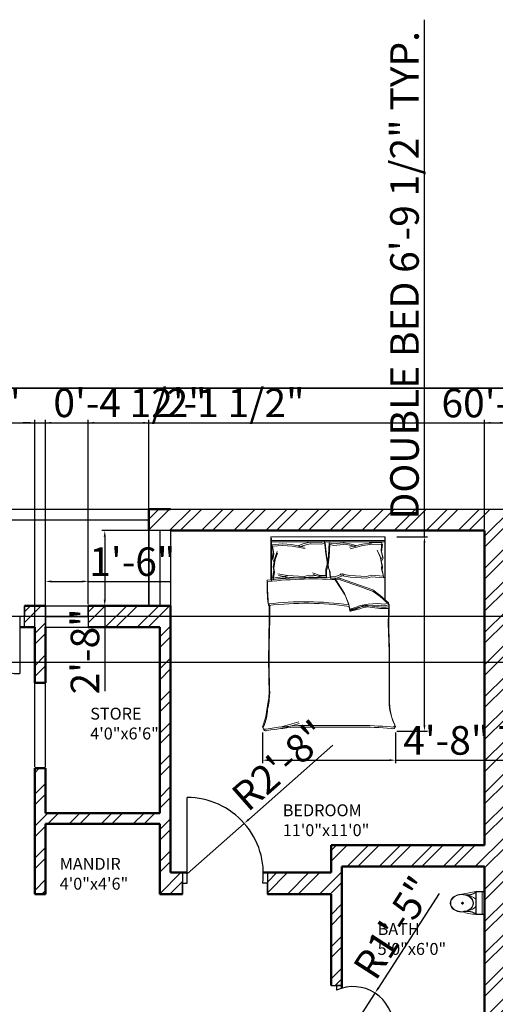
# Model space of a CAD drawing. Units: inches. Extents: x 1990 to 2869, y 1755 to 2533.
# Tile 3 of 6: x 2216 to 2415, y 2120 to 2533. Entities that reach past the tile are written whole.
import ezdxf

# ---------------------------------------------------------------- set-up
doc = ezdxf.new("R2010")
doc.units = ezdxf.units.IN
for name, color, linetype, lineweight in [('A-ANNO-DIMS', 171, 'Continuous', 18), ('A-ANNO-TTLB', 7, 'Continuous', 35), ('A-AREA-IDEN', 7, 'Continuous', 18), ('A-DOOR', 11, 'Continuous', 25), ('A-FLOR-FIXT', 9, 'Continuous', 20), ('A-FURN', 8, 'Continuous', 18), ('A-GLAZ', 121, 'Continuous', 25), ('A-WALL', 7, 'Continuous', 50), ('A-WALL-SITE', 7, 'Continuous', 30)]:
    doc.layers.add(name, color=color, linetype=linetype, lineweight=lineweight)
doc.layers.add('A-WALL-PATT', color=215, linetype='Continuous', lineweight=13, true_color=0xa953a0)
doc.styles.get("Standard").update_dxf_attribs({"font": 'arial.ttf'})
doc.dimstyles.new('ISO-25', dxfattribs={"dimtxt": 12, "dimasz": 2.5, "dimexe": 1.25, "dimexo": 0.625, "dimtad": 1, "dimdec": 0, "dimlunit": 3, "dimtxsty": 'Standard', "dimcen": 2.5, "dimadec": 0, "dimazin": 0, "dimtfac": 1, "dimtdec": 0, "dimtmove": 0, "dimatfit": 3, "dimfxl": 1, "dimarcsym": 0})

# ---------------------------------------------------------------- blocks, each defined once
blk = doc.blocks.new('A$C31115884')
for p, q in [((283, 498), (223, 498)), ((258, 466), (258, 523)), ((0, 200), (0, 0)), ((520, 200), (0, 200)), ((510, 54), (0, 54)), ((10, 190), (10, 10)), ((510, 190), (10, 190)), ((10, 10), (510, 10)), ((510, 10), (510, 190)), ((520, 0), (520, 200)), ((0, 0), (520, 0))]:
    blk.add_line(p, q)
blk.add_circle((256, 496), 23.6)
for centre, radius, start, end in [((2778, -205), 2807, 165.4549, 171.7133), ((-295, 403), 365, 324.2091, 9.3499), ((-295, 403), 375, 324.2091, 9.3499), ((806, 403), 365, 170.6501, 215.7909), ((3237, 905), 2807, 188.2867, 194.5451), ((384, 406), 293, 190.2774, 224.1564), ((139, 406), 293, 315.8436, 2.6563), ((806, 403), 375, 179.2036, 215.7909)]:
    blk.add_arc(centre, radius, start, end)
blk.add_ellipse((256, 510), major_axis=(0, -261), ratio=0.772727)
blk.add_open_spline([(256, 259), (263, 259), (270, 260), (288, 262), (299, 265), (320, 273), (330, 278), (350, 291), (360, 299), (378, 316), (386, 326), (402, 347), (409, 358), (421, 383), (427, 395), (436, 422), (440, 436), (445, 465), (447, 480), (448, 509), (448, 524), (445, 553), (443, 568), (436, 596), (432, 610), (422, 636), (416, 649), (402, 672), (395, 683), (379, 703), (370, 712), (351, 728), (341, 735), (321, 746), (310, 751), (289, 757), (278, 759), (256, 761), (245, 761), (223, 757), (212, 754), (191, 746), (181, 741), (161, 728), (151, 720), (133, 703), (125, 693), (110, 672), (103, 660), (90, 636), (85, 623), (76, 596), (72, 582), (67, 553), (66, 538), (64, 509), (65, 494), (68, 465), (70, 450), (77, 422), (81, 408), (91, 382), (97, 370), (111, 346), (118, 335), (135, 316), (144, 307), (162, 291), (172, 284), (193, 273), (203, 269), (225, 262), (236, 260), (250, 259), (253, 259), (256, 259)], degree=3, knots=[0, 0, 0, 0, 0.110105, 0.110105, 0.285049, 0.285049, 0.459994, 0.459994, 0.634938, 0.634938, 0.809882, 0.809882, 0.984827, 0.984827, 1.159771, 1.159771, 1.334715, 1.334715, 1.50966, 1.50966, 1.684604, 1.684604, 1.859549, 1.859549, 2.034493, 2.034493, 2.209437, 2.209437, 2.384382, 2.384382, 2.559326, 2.559326, 2.73427, 2.73427, 2.909215, 2.909215, 3.084159, 3.084159, 3.259103, 3.259103, 3.434048, 3.434048, 3.608992, 3.608992, 3.783936, 3.783936, 3.958881, 3.958881, 4.133825, 4.133825, 4.30877, 4.30877, 4.483714, 4.483714, 4.658658, 4.658658, 4.833603, 4.833603, 5.008547, 5.008547, 5.183491, 5.183491, 5.358436, 5.358436, 5.53338, 5.53338, 5.708324, 5.708324, 5.883269, 5.883269, 6.058213, 6.058213, 6.233158, 6.233158, 6.283185, 6.283185, 6.283185, 6.283185])
blk = doc.blocks.new('*D3')
at = {"layer": 'A-ANNO-DIMS', "color": 0, "lineweight": -2, "transparency": 16777216}
for p, q in [((2269.35, 2319.05), (2250.15, 2319.05)), ((2251.4, 2316.55), (2251.4, 2290.05)), ((2269.35, 2287.55), (2250.15, 2287.55)), ((2251.4, 2287.55), (2251.4, 2251.7))]:
    blk.add_line(p, q, dxfattribs=at)
at = {"layer": 'A-ANNO-DIMS', "color": 0, "transparency": 16777216}
for points in [[(2250.98, 2316.55), (2251.81, 2316.55), (2251.4, 2319.05)], [(2250.98, 2290.05), (2251.81, 2290.05), (2251.4, 2287.55)]]:
    blk.add_solid(points, dxfattribs=at)
at = {"layer": 'Defpoints', "color": 0, "transparency": 16777216}
for p in [(2269.97, 2319.05), (2251.4, 2287.55), (2269.97, 2287.55)]:
    blk.add_point(p, dxfattribs=at)
at = {"layer": 'A-ANNO-DIMS', "color": 0, "transparency": 16777216, "insert": (2244.64, 2268.37), "char_height": 12, "attachment_point": 5, "rotation": 90}
blk.add_mtext('2\'-8"', dxfattribs=at)
blk = doc.blocks.new('*D4')
at = {"layer": 'A-ANNO-DIMS', "color": 0, "lineweight": -2, "transparency": 16777216}
for p, q in [((2226.47, 2288.18), (2226.47, 2299)), ((2228.97, 2297.75), (2241.97, 2297.75)), ((2244.47, 2288.18), (2244.47, 2299)), ((2244.47, 2297.75), (2278.99, 2297.75))]:
    blk.add_line(p, q, dxfattribs=at)
at = {"layer": 'A-ANNO-DIMS', "color": 0, "transparency": 16777216}
for points in [[(2228.97, 2298.17), (2228.97, 2297.33), (2226.47, 2297.75)], [(2241.97, 2298.17), (2241.97, 2297.33), (2244.47, 2297.75)]]:
    blk.add_solid(points, dxfattribs=at)
at = {"layer": 'Defpoints', "color": 0, "transparency": 16777216}
for p in [(2244.47, 2297.75), (2226.47, 2287.55), (2244.47, 2287.55)]:
    blk.add_point(p, dxfattribs=at)
at = {"layer": 'A-ANNO-DIMS', "color": 0, "transparency": 16777216, "insert": (2262.98, 2304.5), "char_height": 12, "attachment_point": 5}
blk.add_mtext('1\'-6"', dxfattribs=at)
blk = doc.blocks.new('BED-DOUBLE')
for p, q in [((3.47, 63.33), (3.47, 81.44)), ((3.47, 81.44), (51.49, 81.44)), ((3.47, 79.91), (51.27, 79.91)), ((3.48, 63.33), (3.48, 81.44)), ((3.48, 79.91), (51.27, 79.91)), ((3.7, 62.69), (3.7, 80.8)), ((3.7, 62.69), (3.7, 80.8)), ((3.7, 79.27), (51.49, 79.27)), ((3.7, 79.27), (51.49, 79.27)), ((16.88, 78.42), (19.77, 79.14)), ((16.88, 78.42), (19.77, 79.14)), ((19.77, 79.14), (20.09, 79.14)), ((19.77, 79.14), (20.09, 79.14)), ((20.09, 79.14), (24.54, 78.99)), ((20.09, 79.14), (24.54, 78.99)), ((24.54, 78.99), (25.98, 79.57)), ((24.54, 78.99), (25.98, 79.57)), ((24.77, 78.36), (26.21, 78.93)), ((24.77, 78.36), (26.21, 78.93)), ((25.98, 79.57), (26.56, 74.22)), ((25.98, 79.57), (26.56, 74.22)), ((26.21, 78.93), (26.79, 73.58)), ((26.21, 78.93), (26.79, 73.58)), ((27.98, 78.95), (27.73, 73.58)), ((27.98, 78.95), (27.73, 73.58)), ((29.46, 78.46), (27.98, 78.95)), ((29.46, 78.46), (27.98, 78.95)), ((33.88, 78.89), (29.46, 78.46)), ((33.88, 78.89), (29.46, 78.46)), ((34.2, 78.91), (33.88, 78.89)), ((34.2, 78.91), (33.88, 78.89)), ((37.14, 78.36), (34.2, 78.91)), ((37.13, 78.36), (34.2, 78.91)), ((45.71, 78.9), (41.91, 78.37)), ((45.71, 78.9), (41.91, 78.37)), ((50.11, 78.89), (44.71, 78.98)), ((44.71, 78.98), (45.71, 78.9)), ((50.11, 78.89), (44.71, 78.98)), ((44.71, 78.98), (45.71, 78.9)), ((50.11, 78.89), (49.73, 75.68)), ((50.11, 78.89), (49.73, 75.68)), ((51.27, 81.44), (51.27, 54.83)), ((51.27, 81.44), (51.27, 54.83)), ((51.49, 81.44), (51.49, 80.8)), ((51.49, 80.8), (51.49, 54.19)), ((51.49, 80.8), (51.49, 54.19)), ((3.89, 78.13), (4.47, 74.95)), ((3.89, 78.13), (4.47, 74.95)), ((3.9, 78.11), (8.18, 78.43)), ((3.9, 78.11), (8.18, 78.43)), ((4.47, 74.95), (4.04, 72.34)), ((4.47, 74.95), (4.04, 72.34)), ((4.12, 77.49), (4.7, 74.31)), ((4.12, 77.49), (4.7, 74.31)), ((4.13, 77.47), (8.41, 77.8)), ((4.13, 77.47), (8.41, 77.8)), ((5.05, 72.49), (6.06, 75.24)), ((5.05, 72.49), (6.06, 75.24)), ((5.28, 71.85), (6.29, 74.6)), ((5.28, 71.85), (6.29, 74.6)), ((8.18, 78.43), (8.28, 78.42)), ((8.18, 78.43), (8.28, 78.42)), ((8.28, 78.42), (12.11, 78.13)), ((8.28, 78.42), (12.11, 78.13)), ((8.41, 77.8), (8.51, 77.78)), ((8.41, 77.8), (8.51, 77.78)), ((8.51, 77.78), (12.34, 77.49)), ((8.51, 77.78), (12.34, 77.49)), ((12.11, 78.13), (17.6, 77.11)), ((12.11, 78.13), (17.6, 77.11)), ((12.34, 77.49), (17.83, 76.48)), ((12.34, 77.49), (17.83, 76.48)), ((14.85, 77.69), (16.88, 78.42)), ((14.85, 77.69), (16.88, 78.42)), ((15.08, 77.05), (17.11, 77.78)), ((15.08, 77.05), (17.11, 77.78)), ((17.11, 77.78), (20, 78.5)), ((17.11, 77.78), (20, 78.5)), ((20, 78.5), (20.32, 78.5)), ((20, 78.5), (20.32, 78.5)), ((20.32, 78.5), (24.77, 78.36)), ((20.32, 78.5), (24.77, 78.36)), ((28.21, 78.31), (27.96, 72.94)), ((28.2, 78.31), (27.96, 72.94)), ((29.68, 77.82), (28.2, 78.31)), ((29.68, 77.82), (28.21, 78.31)), ((34.11, 78.25), (29.68, 77.82)), ((34.11, 78.25), (29.68, 77.82)), ((34.43, 78.27), (34.11, 78.25)), ((34.43, 78.27), (34.11, 78.25)), ((37.36, 77.73), (34.43, 78.27)), ((37.36, 77.73), (34.43, 78.27)), ((41.91, 78.37), (36.49, 77.02)), ((41.91, 78.37), (36.49, 77.02)), ((42.14, 77.73), (36.72, 76.38)), ((42.14, 77.73), (36.72, 76.38)), ((39.2, 77.77), (37.13, 78.36)), ((39.2, 77.77), (37.14, 78.36)), ((39.43, 77.13), (37.36, 77.73)), ((39.43, 77.13), (37.36, 77.73)), ((45.94, 78.26), (42.14, 77.73)), ((45.94, 78.26), (42.14, 77.73)), ((50.34, 78.25), (44.94, 78.34)), ((44.94, 78.34), (45.94, 78.26)), ((50.34, 78.25), (44.94, 78.34)), ((44.94, 78.34), (45.94, 78.26)), ((49.31, 73.19), (48.13, 75.86)), ((49.31, 73.19), (48.13, 75.86)), ((49.54, 72.55), (48.36, 75.23)), ((49.54, 72.55), (48.36, 75.23)), ((49.73, 75.68), (50.33, 73.1)), ((49.73, 75.68), (50.33, 73.1)), ((50.34, 78.25), (49.96, 75.04)), ((50.34, 78.25), (49.96, 75.04)), ((49.96, 75.04), (50.56, 72.47)), ((49.96, 75.04), (50.56, 72.47)), ((4.04, 72.34), (4.62, 71.33)), ((4.04, 72.34), (4.62, 71.33)), ((4.7, 74.31), (4.27, 71.7)), ((4.7, 74.31), (4.27, 71.7)), ((4.27, 71.7), (4.85, 70.69)), ((4.27, 71.7), (4.85, 70.69)), ((4.47, 68.87), (5.05, 72.49)), ((4.47, 68.87), (5.05, 72.49)), ((4.7, 68.23), (5.28, 71.85)), ((4.7, 68.23), (5.28, 71.85)), ((26.56, 74.22), (27.14, 71.04)), ((26.56, 74.22), (27.14, 71.04)), ((26.79, 73.58), (27.37, 70.4)), ((26.79, 73.58), (27.37, 70.4)), ((27.14, 71.04), (27.14, 69.74)), ((27.14, 71.04), (27.14, 69.74)), ((27.73, 73.58), (27.35, 70.37)), ((27.73, 73.58), (27.35, 70.37)), ((27.35, 70.37), (27.44, 69.07)), ((27.35, 70.37), (27.44, 69.07)), ((27.37, 70.4), (27.37, 69.1)), ((27.37, 70.4), (27.37, 69.1)), ((27.96, 72.94), (27.58, 69.73)), ((27.96, 72.94), (27.58, 69.73)), ((50.11, 69.61), (49.31, 73.19)), ((50.11, 69.61), (49.31, 73.19)), ((50.34, 68.98), (49.54, 72.55)), ((50.34, 68.98), (49.54, 72.55)), ((50.33, 73.1), (49.81, 72.06)), ((50.33, 73.1), (49.81, 72.06)), ((50.56, 72.47), (50.04, 71.42)), ((50.56, 72.47), (50.04, 71.42)), ((4.18, 64.1), (4.76, 67.28)), ((4.18, 64.1), (4.76, 67.28)), ((4.41, 63.46), (4.99, 66.64)), ((4.41, 63.46), (4.99, 66.64)), ((4.76, 67.28), (4.47, 68.87)), ((4.76, 67.28), (4.47, 68.87)), ((4.99, 66.64), (4.7, 68.23)), ((4.99, 66.64), (4.7, 68.23)), ((24.1, 65.18), (20.96, 66.27)), ((24.1, 65.18), (20.96, 66.27)), ((27.14, 69.74), (26.56, 67.86)), ((27.14, 69.74), (26.56, 67.86)), ((26.56, 67.86), (26.56, 65.18)), ((26.56, 67.86), (26.56, 65.18)), ((27.37, 69.1), (26.79, 67.22)), ((27.37, 69.1), (26.79, 67.22)), ((26.79, 67.22), (26.79, 64.54)), ((26.79, 67.22), (26.79, 64.54)), ((27.44, 69.07), (28.13, 67.23)), ((27.44, 69.07), (28.13, 67.23)), ((27.58, 69.73), (27.66, 68.43)), ((27.58, 69.73), (27.66, 68.43)), ((27.66, 68.43), (28.36, 66.59)), ((27.66, 68.43), (28.36, 66.59)), ((28.13, 67.23), (28.3, 64.55)), ((28.13, 67.23), (28.3, 64.55)), ((28.36, 66.59), (28.53, 63.91)), ((28.36, 66.59), (28.53, 63.91)), ((49.92, 68.01), (50.11, 69.61)), ((49.92, 68.01), (50.11, 69.61)), ((50.7, 64.87), (49.92, 68.01)), ((50.7, 64.87), (49.92, 68.01)), ((50.15, 67.37), (50.34, 68.98)), ((50.15, 67.37), (50.34, 68.98)), ((50.93, 64.23), (50.15, 67.37)), ((50.93, 64.23), (50.15, 67.37)), ((9.28, 64.82), (4.18, 64.1)), ((9.28, 64.82), (4.18, 64.1)), ((9.51, 64.19), (4.41, 63.46)), ((9.51, 64.19), (4.41, 63.46)), ((6.38, 65.81), (10.41, 65.15)), ((6.38, 65.81), (10.41, 65.15)), ((6.61, 65.18), (10.64, 64.51)), ((6.61, 65.18), (10.64, 64.51)), ((10.41, 65.15), (9.28, 64.82)), ((10.41, 65.15), (9.28, 64.82)), ((10.64, 64.51), (9.51, 64.19)), ((10.64, 64.51), (9.51, 64.19)), ((10.41, 65.15), (17.42, 64.72)), ((10.41, 65.15), (17.42, 64.72)), ((10.64, 64.51), (17.65, 64.08)), ((10.64, 64.51), (17.65, 64.08)), ((17.42, 64.72), (19.38, 65.27)), ((17.42, 64.72), (19.38, 65.27)), ((17.65, 64.08), (19.61, 64.63)), ((17.65, 64.08), (19.61, 64.63)), ((19.38, 65.27), (24.52, 64.87)), ((19.38, 65.27), (24.52, 64.87)), ((19.61, 64.63), (24.74, 64.23)), ((19.61, 64.63), (24.74, 64.23)), ((24.33, 64.54), (21.19, 65.63)), ((24.33, 64.54), (21.19, 65.63)), ((26.56, 65.18), (24.1, 65.18)), ((26.56, 65.18), (24.1, 65.18)), ((26.79, 64.54), (24.33, 64.54)), ((26.79, 64.54), (24.33, 64.54)), ((28.3, 64.55), (30.75, 64.7)), ((28.3, 64.55), (30.75, 64.7)), ((28.53, 63.91), (30.98, 64.06)), ((28.53, 63.91), (30.98, 64.06)), ((30.26, 64.06), (34.45, 57.57)), ((30.26, 64.06), (34.45, 57.57)), ((30.49, 63.42), (34.68, 56.93)), ((30.49, 63.42), (34.68, 56.93)), ((30.75, 64.7), (33.82, 65.99)), ((30.75, 64.7), (33.82, 65.99)), ((30.98, 64.06), (34.05, 65.35)), ((30.98, 64.06), (34.05, 65.35)), ((40.64, 61.13), (32.31, 64.06)), ((40.64, 61.13), (32.31, 64.06)), ((40.87, 60.49), (32.53, 63.42)), ((40.87, 60.49), (32.53, 63.42)), ((32.56, 65.81), (36.6, 65.15)), ((32.56, 65.81), (36.6, 65.15)), ((32.79, 65.18), (36.82, 64.51)), ((32.79, 65.18), (36.82, 64.51)), ((36.6, 65.15), (43.61, 64.72)), ((36.6, 65.15), (43.61, 64.72)), ((36.82, 64.51), (43.83, 64.08)), ((36.82, 64.51), (43.83, 64.08)), ((43.61, 64.72), (45.57, 65.27)), ((43.61, 64.72), (45.57, 65.27)), ((43.83, 64.08), (45.79, 64.63)), ((43.83, 64.08), (45.79, 64.63)), ((45.57, 65.27), (50.7, 64.87)), ((45.57, 65.27), (50.7, 64.87)), ((45.79, 64.63), (50.93, 64.23)), ((45.79, 64.63), (50.93, 64.23)), ((46.22, 59.11), (40.64, 61.13)), ((46.22, 59.11), (40.64, 61.13)), ((46.45, 58.48), (40.87, 60.49)), ((46.45, 58.48), (40.87, 60.49)), ((49.16, 56.95), (46.22, 59.11)), ((49.16, 56.95), (46.22, 59.11)), ((49.39, 56.31), (46.45, 58.48)), ((49.39, 56.31), (46.45, 58.48)), ((34.45, 57.57), (36.15, 53.08)), ((34.45, 57.57), (36.15, 53.08)), ((34.68, 56.93), (36.38, 52.44)), ((34.68, 56.93), (36.38, 52.44)), ((52.87, 53.7), (49.16, 56.95)), ((52.87, 53.7), (49.16, 56.95)), ((53.1, 53.06), (49.39, 56.31)), ((53.1, 53.06), (49.39, 56.31)), ((36.15, 53.08), (36.46, 51.07)), ((36.15, 53.08), (36.46, 51.07)), ((36.38, 52.44), (36.69, 50.43)), ((36.38, 52.44), (36.69, 50.43)), ((36.46, 51.07), (38.94, 51.69)), ((36.46, 51.07), (38.94, 51.69)), ((36.69, 50.43), (39.17, 51.05)), ((36.69, 50.43), (39.17, 51.05)), ((38.94, 51.69), (40.95, 52.61)), ((38.94, 51.69), (40.95, 52.61)), ((39.17, 51.05), (41.18, 51.97)), ((39.17, 51.05), (41.18, 51.97)), ((40.95, 52.61), (44.36, 53.08)), ((40.95, 52.61), (44.36, 53.08)), ((41.18, 51.97), (44.59, 52.44)), ((41.18, 51.97), (44.59, 52.44)), ((44.36, 53.08), (48.23, 53.39)), ((44.36, 53.08), (48.23, 53.39)), ((44.59, 52.44), (48.46, 52.75)), ((44.59, 52.44), (48.46, 52.75)), ((48.23, 53.39), (51.33, 53.08)), ((48.23, 53.39), (51.33, 53.08)), ((48.46, 52.75), (51.56, 52.44)), ((48.46, 52.75), (51.56, 52.44)), ((51.33, 53.08), (52.87, 53.7)), ((51.33, 53.08), (52.87, 53.7)), ((51.56, 52.44), (53.1, 53.06)), ((51.56, 52.44), (53.1, 53.06)), ((52.95, 51.95), (52.87, 53.7, 3.87)), ((52.95, 51.95), (52.87, 53.7, 3.87)), ((53.18, 51.31), (53.1, 53.06, 3.87)), ((53.18, 51.31), (53.1, 53.06, 3.87)), ((15.06, 2.2), (39.68, 2.2)), ((15.06, 2.2), (39.68, 2.2)), ((15.29, 1.56), (39.91, 1.56)), ((15.29, 1.56), (39.91, 1.56))]:
    blk.add_line(p, q)
for centre, radius, start, end in [((85.16, 61.35), 83.31, 178.7218, 185.604), ((85.16, 61.35), 83.31, 178.7218, 185.604), ((21.36, -100.61), 164.97, 86.0865, 96.7821), ((21.36, -100.61), 164.97, 86.0865, 96.7821), ((85.39, 60.71), 83.31, 178.7218, 185.604), ((85.39, 60.71), 83.31, 178.7218, 185.604), ((21.59, -101.25), 164.97, 86.0865, 96.7821), ((21.59, -101.25), 164.97, 86.0865, 96.7821), ((17.76, -74.87), 129.02, 81.7845, 96.9006), ((17.76, -74.87), 129.02, 81.7845, 96.9006), ((17.98, -75.51), 129.02, 81.7845, 96.9006), ((17.98, -75.51), 129.02, 81.7845, 96.9006), ((-167.31, 50.27), 170.11, 358.4762, 1.0082), ((-167.31, 50.27), 170.11, 358.4762, 1.0082), ((-167.08, 49.63), 170.11, 358.4762, 1.0082), ((-167.08, 49.63), 170.11, 358.4762, 1.0082), ((36.64, 51), 0.185, 160.2464, 271.1377), ((36.64, 51), 0.185, 160.2464, 271.1377), ((31.15, 79.96), 29.65, 280.6617, 289.8806), ((31.15, 79.96), 29.65, 280.6617, 289.8806), ((36.86, 50.36), 0.185, 160.2464, 271.1377), ((36.86, 50.36), 0.185, 160.2464, 271.1377), ((31.38, 79.32), 29.65, 280.6617, 289.8806), ((31.38, 79.32), 29.65, 280.6617, 289.8806), ((43.74, 46.38), 6.22, 78.6608, 113.7384), ((43.74, 46.38), 6.22, 78.6608, 113.7384), ((43.97, 45.74), 6.22, 78.6608, 113.7384), ((43.97, 45.74), 6.22, 78.6608, 113.7384), ((51.33, 88.1), 36.18, 259.8763, 272.5657), ((51.33, 88.1), 36.18, 259.8763, 272.5657), ((51.56, 87.46), 36.18, 259.8763, 272.5657), ((51.56, 87.46), 36.18, 259.8763, 272.5657), ((182.27, 45.13), 129.5, 176.9791, 183.8365), ((182.27, 45.13), 129.5, 176.9791, 183.8365), ((182.49, 44.49), 129.5, 176.9791, 183.8365), ((182.49, 44.49), 129.5, 176.9791, 183.8365), ((484.82, 30.83), 482.31, 178.2277, 181.7185), ((484.82, 30.83), 482.31, 178.2277, 181.7185), ((485.05, 30.19), 482.31, 178.2277, 181.7185), ((485.05, 30.19), 482.31, 178.2277, 181.7185), ((-4508.74, 13.62), 4561.86, 0.00217, 0.28689), ((-4508.74, 13.62), 4561.86, 0.00217, 0.28689), ((-4508.52, 12.98), 4561.86, 0.00217, 0.28689), ((-4508.52, 12.98), 4561.86, 0.00217, 0.28689), ((-26.9, 16.93), 29.63, 346.0648, 358.9113), ((-26.9, 16.93), 29.63, 346.0648, 358.9113), ((-26.67, 16.29), 29.63, 346.0648, 358.9113), ((-26.67, 16.29), 29.63, 346.0648, 358.9113), ((76.16, 12.78), 23.07, 177.4714, 206.4681), ((76.16, 12.78), 23.07, 177.4714, 206.4681), ((76.39, 12.14), 23.07, 177.4714, 206.4681), ((76.39, 12.14), 23.07, 177.4714, 206.4681), ((-21.66, 11.17), 23.56, 337.9751, 356.652), ((-21.66, 11.17), 23.56, 337.9751, 356.652), ((-21.43, 10.53), 23.56, 337.9751, 356.652), ((-21.43, 10.53), 23.56, 337.9751, 356.652), ((1.09, 1.73), 1.09, 146.1736, 293.4781), ((1.09, 1.73), 1.09, 146.1736, 293.4781), ((1.32, 1.09), 1.09, 146.1736, 293.4781), ((1.32, 1.09), 1.09, 146.1736, 293.4781), ((21.43, -119.39), 121.76, 92.9958, 99.4091), ((21.43, -119.39), 121.76, 92.9958, 99.4091), ((21.66, -120.03), 121.76, 92.9958, 99.4091), ((21.65, -120.03), 121.76, 92.9958, 99.4091), ((-17.22, 105.15), 106.46, 283.3832, 287.7053), ((-17.22, 105.15), 106.46, 283.3832, 287.7053), ((-16.99, 104.52), 106.46, 283.3832, 287.7053), ((-16.99, 104.52), 106.46, 283.3832, 287.7053), ((41.15, -130.83), 133.04, 84.4998, 90.6351), ((41.15, -130.83), 133.04, 84.4998, 90.6351), ((41.38, -131.47), 133.04, 84.4998, 90.6351), ((41.38, -131.47), 133.04, 84.4998, 90.6351), ((54.41, 2.57), 1.1, 242.6588, 356.02), ((54.41, 2.57), 1.1, 242.6588, 356.02), ((54.64, 1.93), 1.1, 242.6588, 356.02), ((54.64, 1.93), 1.1, 242.6588, 356.02)]:
    blk.add_arc(centre, radius, start, end)
blk = doc.blocks.new('*D20')
at = {"layer": 'A-ANNO-DIMS', "color": 0, "lineweight": -2, "transparency": 16777216}
for p, q in [((2385.7, 2316.5), (2385.7, 2533.49)), ((2374.09, 2316.5), (2386.95, 2316.5)), ((2385.7, 2237.45), (2385.7, 2314)), ((2374.09, 2234.95), (2386.95, 2234.95))]:
    blk.add_line(p, q, dxfattribs=at)
at = {"layer": 'A-ANNO-DIMS', "color": 0, "transparency": 16777216}
for points in [[(2385.29, 2314), (2386.12, 2314), (2385.7, 2316.5)], [(2385.29, 2237.45), (2386.12, 2237.45), (2385.7, 2234.95)]]:
    blk.add_solid(points, dxfattribs=at)
at = {"layer": 'Defpoints', "color": 0, "transparency": 16777216}
for p in [(2373.47, 2316.5), (2385.7, 2316.5), (2373.47, 2234.95)]:
    blk.add_point(p, dxfattribs=at)
at = {"layer": 'A-ANNO-DIMS', "color": 0, "transparency": 16777216, "insert": (2378.87, 2426.24), "char_height": 12, "attachment_point": 5, "rotation": 90}
blk.add_mtext('DOUBLE BED 6\'-9 1/2" TYP.', dxfattribs=at)
blk = doc.blocks.new('*D21')
at = {"layer": 'A-ANNO-DIMS', "color": 0, "lineweight": -2, "transparency": 16777216}
for p, q in [((2317.65, 2234.33), (2317.65, 2221.47)), ((2373.47, 2234.33), (2373.47, 2221.47)), ((2320.15, 2222.72), (2370.97, 2222.72)), ((2373.47, 2222.72), (2450.85, 2222.72))]:
    blk.add_line(p, q, dxfattribs=at)
at = {"layer": 'A-ANNO-DIMS', "color": 0, "transparency": 16777216}
for points in [[(2320.15, 2223.14), (2320.15, 2222.31), (2317.65, 2222.72)], [(2370.97, 2223.14), (2370.97, 2222.31), (2373.47, 2222.72)]]:
    blk.add_solid(points, dxfattribs=at)
at = {"layer": 'Defpoints', "color": 0, "transparency": 16777216}
for p in [(2317.65, 2234.95), (2373.47, 2234.95), (2373.47, 2222.72)]:
    blk.add_point(p, dxfattribs=at)
at = {"layer": 'A-ANNO-DIMS', "color": 0, "transparency": 16777216, "insert": (2413.41, 2229.47), "char_height": 12, "attachment_point": 5}
blk.add_mtext('4\'-8" TYP.', dxfattribs=at)
blk = doc.blocks.new('*D23')
at = {"layer": 'A-ANNO-DIMS', "color": 0, "lineweight": -2, "transparency": 16777216}
for p, q in [((2435.03, 2169.19), (2437.82, 2169.19)), ((2436.57, 2166.69), (2436.57, 2161.95)), ((2435.03, 2159.45), (2437.82, 2159.45)), ((2436.57, 2159.45), (2436.57, 2054.59))]:
    blk.add_line(p, q, dxfattribs=at)
at = {"layer": 'A-ANNO-DIMS', "color": 0, "transparency": 16777216}
for points in [[(2436.15, 2166.69), (2436.99, 2166.69), (2436.57, 2169.19)], [(2436.15, 2161.95), (2436.99, 2161.95), (2436.57, 2159.45)]]:
    blk.add_solid(points, dxfattribs=at)
at = {"layer": 'Defpoints', "color": 0, "transparency": 16777216}
for p in [(2434.41, 2169.19), (2434.41, 2159.45), (2436.57, 2159.45)]:
    blk.add_point(p, dxfattribs=at)
at = {"layer": 'A-ANNO-DIMS', "color": 0, "transparency": 16777216, "insert": (2429.74, 2105.77), "char_height": 12, "attachment_point": 5, "rotation": 90}
blk.add_mtext('0\'-9 1/2" TYP.', dxfattribs=at)
blk = doc.blocks.new('*D24')
at = {"layer": 'A-ANNO-DIMS', "color": 0, "lineweight": -2, "transparency": 16777216}
for p, q in [((2149.97, 1894.18), (2149.97, 2365.55)), ((2152.47, 2364.3), (2176.34, 2364.3)), ((2178.84, 1894.18), (2178.84, 2365.55)), ((2178.84, 2364.3), (2214.69, 2364.3))]:
    blk.add_line(p, q, dxfattribs=at)
at = {"layer": 'A-ANNO-DIMS', "color": 0, "transparency": 16777216}
for points in [[(2152.47, 2364.72), (2152.47, 2363.88), (2149.97, 2364.3)], [(2176.34, 2364.72), (2176.34, 2363.88), (2178.84, 2364.3)]]:
    blk.add_solid(points, dxfattribs=at)
at = {"layer": 'Defpoints', "color": 0, "transparency": 16777216}
for p in [(2178.84, 2364.3), (2149.97, 1893.55), (2178.84, 1893.55)]:
    blk.add_point(p, dxfattribs=at)
at = {"layer": 'A-ANNO-DIMS', "color": 0, "transparency": 16777216, "insert": (2198.02, 2371.05), "char_height": 12, "attachment_point": 5}
blk.add_mtext('2\'-5"', dxfattribs=at)
blk = doc.blocks.new('*D36')
at = {"layer": 'A-ANNO-DIMS', "color": 0, "lineweight": -2, "transparency": 16777216}
for p, q in [((2716.35, 2283.05), (2016.97, 2283.05)), ((2018.22, 2280.55), (2018.22, 2266.18)), ((2716.35, 2263.68), (2016.97, 2263.68)), ((2018.22, 2263.68), (2018.22, 2201.19))]:
    blk.add_line(p, q, dxfattribs=at)
at = {"layer": 'A-ANNO-DIMS', "color": 0, "transparency": 16777216}
for points in [[(2017.8, 2280.55), (2018.64, 2280.55), (2018.22, 2283.05)], [(2017.8, 2266.18), (2018.64, 2266.18), (2018.22, 2263.68)]]:
    blk.add_solid(points, dxfattribs=at)
at = {"layer": 'Defpoints', "color": 0, "transparency": 16777216}
for p in [(2716.97, 2283.05), (2018.22, 2263.68), (2716.97, 2263.68)]:
    blk.add_point(p, dxfattribs=at)
at = {"layer": 'A-ANNO-DIMS', "color": 0, "transparency": 16777216, "insert": (2011.39, 2231.19), "char_height": 12, "attachment_point": 5, "rotation": 90}
blk.add_mtext('1\'-7 1/2"', dxfattribs=at)
blk = doc.blocks.new('*D37')
at = {"layer": 'A-ANNO-DIMS', "color": 0, "lineweight": -2, "transparency": 16777216}
for p, q in [((2244.47, 2288.18), (2244.47, 2365.55)), ((2246.97, 2364.3), (2267.47, 2364.3)), ((2269.97, 2288.18), (2269.97, 2365.55)), ((2269.97, 2364.3), (2333.79, 2364.3))]:
    blk.add_line(p, q, dxfattribs=at)
at = {"layer": 'A-ANNO-DIMS', "color": 0, "transparency": 16777216}
for points in [[(2246.97, 2364.72), (2246.97, 2363.88), (2244.47, 2364.3)], [(2267.47, 2364.72), (2267.47, 2363.88), (2269.97, 2364.3)]]:
    blk.add_solid(points, dxfattribs=at)
at = {"layer": 'Defpoints', "color": 0, "transparency": 16777216}
for p in [(2269.97, 2364.3), (2244.47, 2287.55), (2269.97, 2287.55)]:
    blk.add_point(p, dxfattribs=at)
at = {"layer": 'A-ANNO-DIMS', "color": 0, "transparency": 16777216, "insert": (2303.13, 2371.13), "char_height": 12, "attachment_point": 5}
blk.add_mtext('2\'-1 1/2"', dxfattribs=at)
blk = doc.blocks.new('*D40')
at = {"layer": 'A-ANNO-DIMS', "color": 0, "lineweight": -2, "transparency": 16777216}
for p, q in [((2410.97, 2319.68), (2410.97, 2365.55)), ((2413.47, 2364.3), (2417.47, 2364.3)), ((2419.97, 2319.68), (2419.97, 2365.55)), ((2419.97, 2364.3), (2455.62, 2364.3))]:
    blk.add_line(p, q, dxfattribs=at)
at = {"layer": 'A-ANNO-DIMS', "color": 0, "transparency": 16777216}
for points in [[(2413.47, 2364.72), (2413.47, 2363.88), (2410.97, 2364.3)], [(2417.47, 2364.72), (2417.47, 2363.88), (2419.97, 2364.3)]]:
    blk.add_solid(points, dxfattribs=at)
at = {"layer": 'Defpoints', "color": 0, "transparency": 16777216}
for p in [(2419.97, 2364.3), (2410.97, 2319.05), (2419.97, 2319.05)]:
    blk.add_point(p, dxfattribs=at)
at = {"layer": 'A-ANNO-DIMS', "color": 0, "transparency": 16777216, "insert": (2439.05, 2371.05), "char_height": 12, "attachment_point": 5}
blk.add_mtext('0\'-9"', dxfattribs=at)
blk = doc.blocks.new('*D41')
at = {"layer": 'A-ANNO-DIMS', "color": 0, "lineweight": -2, "transparency": 16777216}
for p, q in [((2219.47, 2364.3), (2216.97, 2364.3)), ((2221.97, 2219.99), (2221.97, 2365.55)), ((2221.97, 2364.3), (2226.47, 2364.3)), ((2226.47, 2219.99), (2226.47, 2365.55)), ((2228.97, 2364.3), (2292.58, 2364.3))]:
    blk.add_line(p, q, dxfattribs=at)
at = {"layer": 'A-ANNO-DIMS', "color": 0, "transparency": 16777216}
for points in [[(2219.47, 2364.72), (2219.47, 2363.88), (2221.97, 2364.3)], [(2228.97, 2364.72), (2228.97, 2363.88), (2226.47, 2364.3)]]:
    blk.add_solid(points, dxfattribs=at)
at = {"layer": 'Defpoints', "color": 0, "transparency": 16777216}
for p in [(2226.47, 2364.3), (2221.97, 2219.37), (2226.47, 2219.37)]:
    blk.add_point(p, dxfattribs=at)
at = {"layer": 'A-ANNO-DIMS', "color": 0, "transparency": 16777216, "insert": (2262.03, 2371.13), "char_height": 12, "attachment_point": 5}
blk.add_mtext('0\'-4 1/2"', dxfattribs=at)
blk = doc.blocks.new('*D48')
at = {"layer": 'A-ANNO-DIMS', "color": 0, "lineweight": -2, "transparency": 16777216}
for p, q in [((2054.47, 2328.68), (2054.47, 2365.55)), ((2056.97, 2364.3), (2773.97, 2364.3)), ((2776.47, 2328.68), (2776.47, 2365.55))]:
    blk.add_line(p, q, dxfattribs=at)
at = {"layer": 'A-ANNO-DIMS', "color": 0, "transparency": 16777216}
for points in [[(2056.97, 2364.72), (2056.97, 2363.88), (2054.47, 2364.3)], [(2773.97, 2364.72), (2773.97, 2363.88), (2776.47, 2364.3)]]:
    blk.add_solid(points, dxfattribs=at)
at = {"layer": 'Defpoints', "color": 0, "transparency": 16777216}
for p in [(2776.47, 2364.3), (2054.47, 2328.05), (2776.47, 2328.05)]:
    blk.add_point(p, dxfattribs=at)
at = {"layer": 'A-ANNO-DIMS', "color": 0, "transparency": 16777216, "insert": (2415.47, 2371.05), "char_height": 12, "attachment_point": 5}
blk.add_mtext('60\'-2"', dxfattribs=at)
blk = doc.blocks.new('*D54')
at = {"layer": 'A-ANNO-DIMS', "color": 0, "lineweight": -2, "transparency": 16777216}
for p, q in [((2347.24, 2229.05), (2311.89, 2197.87)), ((2286.01, 2175.04), (2310.02, 2196.22))]:
    blk.add_line(p, q, dxfattribs=at)
at = {"layer": 'A-ANNO-DIMS', "color": 0, "transparency": 16777216}
blk.add_solid([(2311.62, 2198.18), (2312.17, 2197.56), (2310.02, 2196.22)], dxfattribs=at)
at = {"layer": 'Defpoints', "color": 0, "transparency": 16777216}
for p in [(2310.02, 2196.22), (2286.01, 2175.04)]:
    blk.add_point(p, dxfattribs=at)
at = {"layer": 'A-ANNO-DIMS', "color": 0, "transparency": 16777216, "insert": (2326.04, 2219.35), "char_height": 12, "attachment_point": 5, "rotation": 41.4179}
blk.add_mtext('R2\'-8"', dxfattribs=at)
blk = doc.blocks.new('*D61')
at = {"layer": 'A-ANNO-DIMS', "color": 0, "lineweight": -2, "transparency": 16777216}
for p, q in [((2391.86, 2166.71), (2366.3, 2127.11)), ((2355.72, 2110.72), (2364.94, 2125.01))]:
    blk.add_line(p, q, dxfattribs=at)
at = {"layer": 'A-ANNO-DIMS', "color": 0, "transparency": 16777216}
blk.add_solid([(2365.95, 2127.34), (2366.65, 2126.88), (2364.94, 2125.01)], dxfattribs=at)
at = {"layer": 'Defpoints', "color": 0, "transparency": 16777216}
for p in [(2364.94, 2125.01), (2355.72, 2110.72)]:
    blk.add_point(p, dxfattribs=at)
at = {"layer": 'A-ANNO-DIMS', "color": 0, "transparency": 16777216, "insert": (2374.09, 2151.62), "char_height": 12, "attachment_point": 5, "rotation": 57.1524}
blk.add_mtext('R1\'-5"', dxfattribs=at)

msp = doc.modelspace()

# ---------------------------------------------------------------- hatches: boundary and pattern name
at = {"layer": 'A-WALL-PATT'}
h = msp.add_hatch(dxfattribs=at)
h.set_pattern_fill('ANSI32', color=256)
h.paths.add_polyline_path([(2193.46, 2287.55), (2131.97, 2287.55), (2131.97, 2278.55), (2193.46, 2278.55)])
h.paths.add_polyline_path([(2113.97, 2278.55), (2113.97, 2287.55), (2104.97, 2287.55), (2104.97, 2257.5), (2113.97, 2257.5)])
h.paths.add_polyline_path([(2113.97, 2205), (2104.97, 2205), (2104.97, 2166.55), (2140.97, 2166.55), (2140.97, 2160.48), (2149.97, 2160.48), (2149.97, 2166.55), (2170.14, 2166.55), (2170.14, 2175.55), (2113.97, 2175.55)])
h.paths.add_polyline_path([(2278.97, 2287.55), (2244.47, 2287.55), (2244.47, 2278.55), (2274.47, 2278.55), (2274.47, 2200.55), (2226.47, 2200.55), (2226.47, 2219.37), (2221.97, 2219.37), (2221.97, 2175.55), (2221.97, 2166.55), (2226.47, 2166.55), (2226.47, 2196.05), (2274.47, 2196.05), (2274.47, 2166.55), (2284.01, 2166.55), (2284.01, 2171.05), (2284.01, 2175.55), (2278.97, 2175.55), (2278.97, 2278.55)])
h.paths.add_polyline_path([(2226.47, 2283.05), (2226.47, 2287.55), (2217.66, 2287.55), (2217.66, 2283.05), (2217.66, 2278.55), (2221.97, 2278.55), (2221.97, 2255.21), (2226.47, 2255.21), (2226.47, 2278.55)])
h.paths.add_polyline_path([(2560.97, 2328.05), (2551.97, 2328.05), (2269.97, 2328.05), (2269.97, 2319.05), (2278.97, 2319.05), (2410.97, 2319.05), (2410.97, 2187.05), (2346.47, 2187.05), (2346.47, 2175.55), (2319.77, 2175.55), (2319.77, 2166.55), (2346.47, 2166.55), (2346.47, 2128.22), (2350.97, 2128.22), (2350.97, 2178.05), (2410.97, 2178.05), (2410.97, 2175.55), (2410.97, 2106.05), (2350.97, 2106.05), (2350.97, 2108.72), (2348.72, 2108.72), (2346.47, 2108.72), (2346.47, 2106.05), (2342.3, 2106.05), (2342.3, 2097.05), (2346.47, 2097.05), (2350.97, 2097.05), (2410.97, 2097.05), (2410.97, 1974.05), (2373.73, 1974.05), (2373.73, 1965.05), (2419.97, 1965.05), (2447.99, 1965.05), (2447.99, 1969.55), (2447.99, 1974.05), (2419.97, 1974.05), (2419.97, 2097.05), (2484.47, 2097.05), (2489.55, 2097.05), (2489.55, 2106.05), (2484.47, 2106.05), (2484.47, 2108.84), (2482.22, 2108.84), (2479.97, 2108.84), (2479.97, 2106.05), (2419.97, 2106.05), (2419.97, 2175.55), (2419.97, 2178.05), (2479.97, 2178.05), (2479.97, 2128.49), (2484.47, 2128.49), (2484.47, 2166.55), (2511.88, 2166.55), (2511.88, 2171.05), (2511.88, 2175.55), (2484.47, 2175.55), (2484.47, 2187.05), (2479.97, 2187.05), (2419.97, 2187.05), (2419.97, 2319.05), (2551.97, 2319.05), (2560.97, 2319.05)])
h.paths.add_polyline_path([(2586.47, 2292.05), (2560.97, 2292.05), (2551.97, 2292.05), (2551.97, 2175.55), (2547.37, 2175.55), (2547.37, 2166.55), (2556.47, 2166.55), (2556.47, 2175.55), (2556.47, 2205.05), (2604.47, 2205.05), (2604.47, 2166.55), (2608.97, 2166.55), (2608.97, 2175.55), (2608.97, 2205.05), (2608.97, 2228.1), (2604.47, 2228.1), (2604.47, 2209.55), (2556.47, 2209.55), (2556.47, 2283.05), (2586.47, 2283.05)])
h.paths.add_polyline_path([(2691.55, 2292.05), (2690.86, 2292.05), (2636.82, 2292.05), (2636.82, 2283.05), (2691.55, 2283.05)])
h.paths.add_polyline_path([(2725.97, 2292.05), (2716.97, 2292.05), (2709.55, 2292.05), (2709.55, 2287.55), (2709.55, 2283.05), (2716.97, 2283.05), (2716.97, 2263.68), (2725.97, 2263.68)])
h.paths.add_polyline_path([(2725.97, 2199.18), (2716.97, 2199.18), (2716.97, 2180.05), (2716.97, 2175.55), (2650.43, 2175.55), (2650.43, 2166.55), (2680.97, 2166.55), (2680.97, 2159.77), (2689.97, 2159.77), (2689.97, 2166.55), (2725.97, 2166.55)])
h.paths.add_polyline_path([(2536.97, 2061.55), (2554.82, 2061.55), (2554.82, 2070.55), (2536.97, 2070.55), (2536.97, 2097.05), (2536.97, 2106.05), (2524.42, 2106.05), (2524.42, 2101.55), (2524.42, 2097.05), (2527.97, 2097.05), (2527.97, 1974.05), (2497.49, 1974.05), (2497.49, 1965.05), (2527.97, 1965.05), (2527.97, 1929.96), (2536.97, 1929.96)])
h.paths.add_polyline_path([(2689.97, 1945.55), (2685.47, 1945.55), (2680.97, 1945.55), (2680.97, 1893.55), (2625.68, 1893.55), (2625.68, 1884.55), (2689.97, 1884.55), (2689.97, 1893.55)])
h.paths.add_polyline_path([(2168.89, 2070.55), (2149.97, 2070.55), (2149.97, 2116.52), (2145.47, 2116.52), (2140.97, 2116.52), (2140.97, 1977.7), (2145.47, 1977.7), (2145.47, 1977.63), (2149.97, 1977.55), (2149.97, 2061.55), (2168.89, 2061.55)])
h.paths.add_polyline_path([(2302.97, 2097.05), (2306.2, 2097.05), (2306.2, 2106.05), (2293.97, 2106.05), (2293.97, 2097.05), (2293.97, 2070.55), (2269.93, 2070.55), (2269.93, 2061.55), (2293.97, 2061.55), (2293.97, 1930.78), (2302.97, 1930.78), (2302.97, 1965.05), (2324.23, 1965.05), (2324.23, 1969.55), (2324.23, 1974.05), (2302.97, 1974.05)])
h.paths.add_polyline_path([(2149.97, 1928.2), (2145.47, 1928.2), (2140.97, 1928.2), (2140.97, 1889.05), (2140.97, 1884.55), (2178.84, 1884.55), (2178.84, 1889.05), (2178.84, 1893.55), (2149.97, 1893.55)])
h.paths.add_polyline_path([(2302.97, 1898.24), (2298.47, 1898.24), (2293.97, 1898.24), (2293.97, 1893.55), (2243.34, 1893.55), (2243.34, 1884.55), (2302.97, 1884.55)])

# ---------------------------------------------------------------- linework, layer by layer
at = {"layer": 'A-ANNO-TTLB'}
msp.add_lwpolyline([(1989.71, 2378.83), (2869.46, 2378.83), (2869.46, 1755.45), (1989.71, 1755.45)], close=True, dxfattribs=at)
at = {"layer": 'A-DOOR'}
for p, q in [((2217.66, 2278.55), (2217.66, 2287.55)), ((2217.66, 2287.55), (2217.66, 2283.05)), ((2217.66, 2283.05), (2215.66, 2283.05)), ((2215.66, 2283.05), (2215.66, 2259.05)), ((2286.01, 2171.05), (2286.01, 2207.05)), ((2284.01, 2175.55), (2284.01, 2166.55)), ((2319.77, 2175.55), (2319.77, 2166.55)), ((2284.01, 2166.55), (2284.01, 2171.05)), ((2284.01, 2171.05), (2286.01, 2171.05)), ((2319.77, 2171.05), (2317.77, 2171.05)), ((2319.77, 2166.55), (2319.77, 2171.05)), ((2346.47, 2128.22), (2350.97, 2128.22)), ((2350.97, 2128.22), (2348.72, 2128.22)), ((2348.72, 2128.22), (2348.72, 2126.22))]:
    msp.add_line(p, q, dxfattribs=at)
for centre, radius, start, end in [((2215.66, 2279.55), 20.5, 170.1581, 270), ((2286.01, 2175.04), 32.01, 352.8352, 90), ((2355.72, 2110.72), 17, 0, 114.3008)]:
    msp.add_arc(centre, radius, start, end, dxfattribs=at)
at = {"layer": 'A-GLAZ'}
for p, q in [((2278.97, 2319.05), (2269.97, 2319.05)), ((2269.97, 2319.05), (2269.97, 2287.55)), ((2274.47, 2319.05), (2274.47, 2287.55)), ((2278.97, 2319.05), (2278.97, 2287.55)), ((2226.47, 2287.55), (2226.47, 2278.55)), ((2226.47, 2287.55), (2244.47, 2287.55)), ((2244.47, 2283.05), (2244.47, 2287.55)), ((2244.47, 2287.55), (2244.47, 2278.55)), ((2226.47, 2278.55), (2226.47, 2283.05)), ((2226.47, 2283.05), (2244.47, 2283.05)), ((2226.47, 2278.55), (2244.47, 2278.55))]:
    msp.add_line(p, q, dxfattribs=at)
at = {"layer": 'A-WALL'}
for p, q in [((2278.97, 2328.05), (2269.97, 2328.05)), ((2269.97, 2328.05), (2269.97, 2319.05)), ((2278.97, 2319.05), (2410.97, 2319.05)), ((2410.97, 2319.05), (2410.97, 2187.05)), ((2217.66, 2287.55), (2226.47, 2287.55)), ((2244.47, 2287.55), (2278.97, 2287.55)), ((2278.97, 2278.55), (2278.97, 2287.55)), ((2215.66, 2278.55), (2221.97, 2278.55)), ((2221.97, 2278.55), (2221.97, 2255.21)), ((2226.47, 2278.55), (2226.47, 2255.21)), ((2244.47, 2278.55), (2274.47, 2278.55)), ((2274.47, 2278.55), (2274.47, 2200.55)), ((2278.97, 2278.55), (2278.97, 2175.55)), ((2221.97, 2255.21), (2226.47, 2255.21)), ((2221.97, 2219.37), (2226.47, 2219.37)), ((2221.97, 2219.37), (2221.97, 2175.55)), ((2226.47, 2219.37), (2226.47, 2200.55)), ((2226.47, 2200.55), (2274.47, 2200.55)), ((2226.47, 2196.05), (2274.47, 2196.05)), ((2226.47, 2196.05), (2226.47, 2166.55)), ((2274.47, 2196.05), (2274.47, 2166.55)), ((2346.47, 2187.05), (2410.97, 2187.05)), ((2350.97, 2187.05), (2346.47, 2187.05)), ((2346.47, 2187.05), (2346.47, 2175.55)), ((2410.97, 2178.05), (2350.97, 2178.05)), ((2350.97, 2178.05), (2350.97, 2127.05)), ((2410.97, 2178.05), (2410.97, 2175.55)), ((2221.97, 2175.55), (2221.97, 2166.55)), ((2278.97, 2175.55), (2286.01, 2175.55)), ((2318.02, 2175.55), (2346.47, 2175.55)), ((2410.97, 2106.05), (2410.97, 2175.55)), ((2221.97, 2166.55), (2226.47, 2166.55)), ((2274.47, 2166.55), (2284.01, 2166.55)), ((2319.77, 2166.55), (2346.47, 2166.55)), ((2346.47, 2128.22), (2346.47, 2166.55))]:
    msp.add_line(p, q, dxfattribs=at)
at = {"layer": 'A-WALL-SITE'}
for p, q in [((2054.47, 2328.05), (2776.47, 2328.05)), ((2058.97, 2323.55), (2269.97, 2323.55))]:
    msp.add_line(p, q, dxfattribs=at)

# ---------------------------------------------------------------- block references
at = {"layer": 'A-FLOR-FIXT', "xscale": 0.0187314124412627, "yscale": 0.0187314124412627, "zscale": 0.0187314124412627, "rotation": 89.99999999999999}
msp.add_blockref('A$C31115884', (2410.97, 2157.93), dxfattribs=at)
at = {"layer": 'A-FURN'}
msp.add_blockref('BED-DOUBLE', (2317.73, 2235.06), dxfattribs=at)

# ---------------------------------------------------------------- texts
at = {"layer": 'A-AREA-IDEN', "char_height": 5, "attachment_point": 1}
for s, width, insert in [('STORE\\P4\'0"x6\'6"', 107.379, (2245.3, 2244.75)), ('BEDROOM\\P11\'0"x11\'0"', 129.7116, (2326.18, 2204.19)), ('MANDIR\\P4\'0"x4\'6"', 73.7331, (2232.47, 2181.72)), ('BATH\\P5\'0"x6\'0"', 161.1281, (2366.03, 2154.35))]:
    msp.add_mtext_dynamic_manual_height_columns(s, width=width, gutter_width=12.5, heights=[0], dxfattribs=dict(at, insert=insert))

# ---------------------------------------------------------------- dimensions: what is measured, and where the dimension line sits
at = {"layer": 'A-ANNO-DIMS'}
for base, p1, p2, angle, text, picture, middle in [((2385.7023, 2316.5031), (2373.47, 2234.9545), (2373.47, 2316.5031), 90, 'DOUBLE BED <> TYP.', '*D20', (2378.8685, 2426.2448)), ((2436.57, 2159.45), (2434.41, 2169.19), (2434.41, 2159.45), 270, '<> TYP.', '*D23', (2429.74, 2105.77))]:
    dim = msp.add_linear_dim(base=base, p1=p1, p2=p2, angle=angle, text=text, dimstyle='ISO-25', override={"dimdec": 1, "dimlfac": 1, "dimrnd": 0, "dimzin": 1, "dimdsep": 46, "dimlunit": 4, "dimfrac": 2}, dxfattribs=at)
    dim.commit()
    dim.dimension.update_dxf_attribs({"geometry": picture, "text_midpoint": middle})
for base, p1, p2, override, picture, middle in [((2226.47, 2364.3), (2221.97, 2219.37), (2226.47, 2219.37), {"dimdec": 1, "dimlfac": 1, "dimrnd": 0, "dimzin": 1, "dimdsep": 46, "dimlunit": 4, "dimfrac": 2}, '*D41', (2262.03, 2371.13)), ((2269.97, 2364.3), (2244.47, 2287.55), (2269.97, 2287.55), {"dimdec": 1, "dimlfac": 1, "dimrnd": 0, "dimzin": 1, "dimdsep": 46, "dimlunit": 4, "dimfrac": 2}, '*D37', (2303.13, 2371.13)), ((2776.47, 2364.3), (2054.47, 2328.05), (2776.47, 2328.05), {"dimdec": 1, "dimlfac": 1, "dimrnd": 0, "dimzin": 1, "dimdsep": 46, "dimlunit": 4, "dimfrac": 2}, '*D48', (2415.47, 2371.05)), ((2178.84, 2364.3), (2149.97, 1893.55), (2178.84, 1893.55), {"dimdec": 1, "dimlfac": 1, "dimrnd": 0, "dimzin": 1, "dimdsep": 46, "dimlunit": 4, "dimfrac": 2}, '*D24', (2198.02, 2371.05)), ((2419.97, 2364.3), (2410.97, 2319.05), (2419.97, 2319.05), {"dimdec": 1, "dimlfac": 1, "dimrnd": 0, "dimzin": 1, "dimdsep": 46, "dimlunit": 4, "dimfrac": 2}, '*D40', (2439.05, 2371.05)), ((2244.47, 2297.75), (2226.47, 2287.55), (2244.47, 2287.55), {"dimclrd": 0, "dimclre": 0, "dimclrt": 0}, '*D4', (2262.98, 2304.5))]:
    dim = msp.add_linear_dim(base=base, p1=p1, p2=p2, dimstyle='ISO-25', override=override, dxfattribs=at)
    dim.commit()
    dim.dimension.update_dxf_attribs({"geometry": picture, "text_midpoint": middle})
for base, p1, p2, override, picture, middle in [((2251.39642545, 2287.55122255), (2269.97134122, 2319.05122255), (2269.97134122, 2287.55122255), {"dimclrd": 0, "dimclre": 0, "dimclrt": 0}, '*D3', (2244.6445496, 2268.3743808)), ((2018.22, 2263.68), (2716.97, 2283.05), (2716.97, 2263.68), {"dimdec": 1, "dimlfac": 1, "dimrnd": 0, "dimzin": 1, "dimdsep": 46, "dimlunit": 4, "dimfrac": 2}, '*D36', (2011.39, 2231.19))]:
    dim = msp.add_linear_dim(base=base, p1=p1, p2=p2, angle=90, dimstyle='ISO-25', override=override, dxfattribs=at)
    dim.commit()
    dim.dimension.update_dxf_attribs({"geometry": picture, "text_midpoint": middle})
dim = msp.add_linear_dim(base=(2373.47, 2222.72), p1=(2317.65, 2234.95), p2=(2373.47, 2234.95), text='<> TYP.', dimstyle='ISO-25', override={"dimdec": 1, "dimlfac": 1, "dimrnd": 0, "dimzin": 1, "dimdsep": 46, "dimlunit": 4, "dimfrac": 2}, dxfattribs=at)
dim.commit()
dim.dimension.update_dxf_attribs({"geometry": '*D21', "text_midpoint": (2413.41, 2229.47)})
for center, mpoint, picture, middle in [((2286.01, 2175.04), (2310.02, 2196.22), '*D54', (2326.04, 2219.35)), ((2355.72, 2110.72), (2364.94, 2125.01), '*D61', (2374.09, 2151.62))]:
    dim = msp.add_radius_dim(center=center, mpoint=mpoint, dimstyle='ISO-25', override={"dimdec": 1, "dimlfac": 1, "dimrnd": 0, "dimzin": 1, "dimdsep": 46, "dimlunit": 4, "dimfrac": 2}, dxfattribs=at)
    dim.commit()
    dim.dimension.update_dxf_attribs({"geometry": picture, "text_midpoint": middle})

doc.saveas('drawing.dxf')
